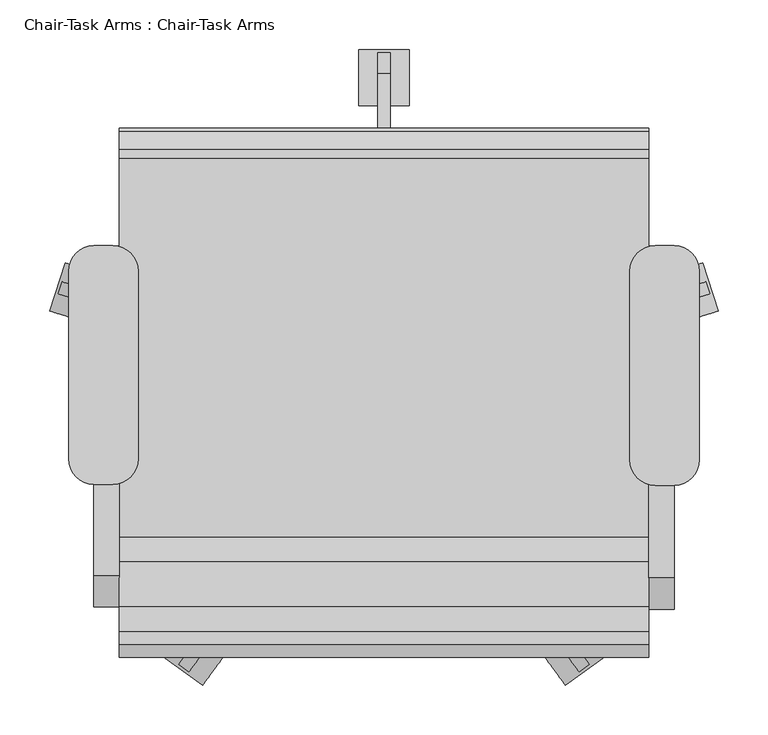
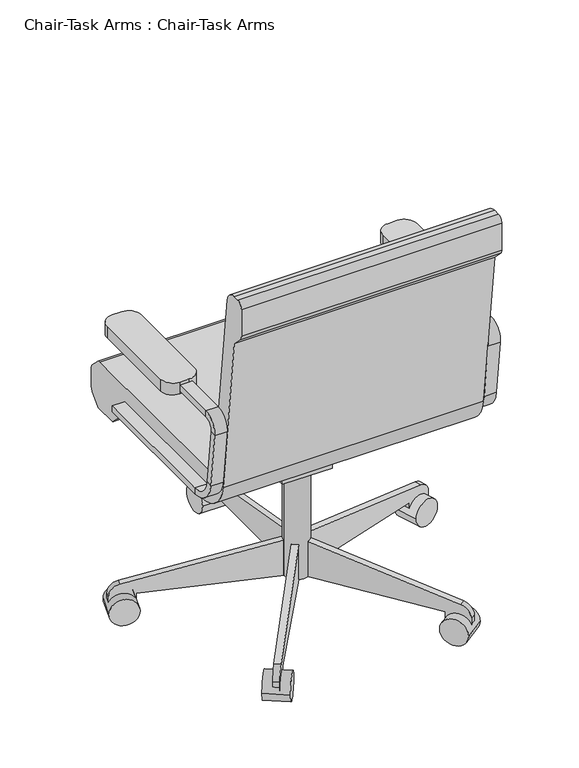
"""IFC4 building model written with IfcOpenShell, lengths in millimetres: furniture geometry, Chair-Task Arms : Chair-Task Arms."""

from ifc_helpers import new_model, si_unit, point, frame, frame_2d, origin, place, context, project, spatial, polyline, circle_curve, trimmed, segment, composite_curve, outline, extrude, source, transform, mapped, element, save
from ifc_brep_helpers import plane_surface, cylinder_surface, revolved_surface, advanced_brep


def chair_task_arms_chair_task_arms_fa5a08ef(model_context):
    return source(origin(), model_context, "Body", "SolidModel", [
        extrude(outline(composite_curve([segment(polyline([(433.0908197, -74.2028048), (414.0408197, -74.2028048)]), True, "CONTINUOUS"), segment(trimmed(circle_curve(frame_2d((414.0408197, -48.8028048)), 25.4), [point((414.0408197, -74.2028048))], [point((388.6408197, -48.8028048))], False, "CARTESIAN"), True, "CONTINUOUS"), segment(polyline([(388.6408197, -48.8028048), (388.6408197, 141.6319091)]), True, "CONTINUOUS"), segment(trimmed(circle_curve(frame_2d((414.0408197, 141.6319091)), 25.4), [point((388.6408197, 141.6319091))], [point((414.0408197, 167.0319091))], False, "CARTESIAN"), True, "CONTINUOUS"), segment(polyline([(414.0408197, 167.0319091), (433.0908197, 167.0319091)]), True, "CONTINUOUS"), segment(trimmed(circle_curve(frame_2d((433.0908197, 141.6319091)), 25.4), [point((433.0908197, 167.0319091))], [point((458.4908197, 141.6319091))], False, "CARTESIAN"), True, "CONTINUOUS"), segment(polyline([(458.4908197, 141.6319091), (458.4908197, -48.8028048)]), True, "CONTINUOUS"), segment(trimmed(circle_curve(frame_2d((433.0908197, -48.8028048)), 25.4), [point((458.4908197, -48.8028048))], [point((433.0908197, -74.2028048))], False, "CARTESIAN"), True, "CONTINUOUS")], self_intersect=False)), frame((0.0, 0.0, 596.9), z_axis=(0.0, 0.0, 1.0), x_axis=(1.0, 0.0, 0.0)), (0.0, 0.0, 1.0), 25.4),
        extrude(outline(composite_curve([segment(polyline([(-132.0591803, -73.1575984), (-151.1091803, -73.1575984)]), True, "CONTINUOUS"), segment(trimmed(circle_curve(frame_2d((-151.1091803, -47.7575984)), 25.4), [point((-151.1091803, -73.1575984))], [point((-176.5091803, -47.7575984))], False, "CARTESIAN"), True, "CONTINUOUS"), segment(polyline([(-176.5091803, -47.7575984), (-176.5091803, 141.6319091)]), True, "CONTINUOUS"), segment(trimmed(circle_curve(frame_2d((-151.1091803, 141.6319091)), 25.4), [point((-176.5091803, 141.6319091))], [point((-151.1091803, 167.0319091))], False, "CARTESIAN"), True, "CONTINUOUS"), segment(polyline([(-151.1091803, 167.0319091), (-132.0591803, 167.0319091)]), True, "CONTINUOUS"), segment(trimmed(circle_curve(frame_2d((-132.0591803, 141.6319091)), 25.4), [point((-132.0591803, 167.0319091))], [point((-106.6591803, 141.6319091))], False, "CARTESIAN"), True, "CONTINUOUS"), segment(polyline([(-106.6591803, 141.6319091), (-106.6591803, -47.7575984)]), True, "CONTINUOUS"), segment(trimmed(circle_curve(frame_2d((-132.0591803, -47.7575984)), 25.4), [point((-106.6591803, -47.7575984))], [point((-132.0591803, -73.1575984))], False, "CARTESIAN"), True, "CONTINUOUS")], self_intersect=False)), frame((0.0, 0.0, 596.9), z_axis=(0.0, 0.0, 1.0), x_axis=(1.0, 0.0, 0.0)), (0.0, 0.0, 1.0), 25.4),
        advanced_brep(
        [(-151.1091803, 167.0319091, 412.75), (-151.1091803, 167.0319091, 425.45), (-125.7091803, 167.0319091, 425.45), (-125.7091803, 167.0319091, 412.75), (-151.1091803, -126.2388651, 412.75), (-151.1091803, -126.2388651, 425.45), (-125.7091803, -126.2388651, 425.45), (-125.7091803, -126.2388651, 412.75), (-151.1091803, -170.3844094, 464.7064065), (-151.1091803, -182.9974221, 463.2225227), (-125.7091803, -170.3844094, 464.7064065), (-125.7091803, -182.9974221, 463.2225227), (-151.1091803, -196.7936301, 580.4902904), (-151.1091803, -184.1806174, 581.9741742), (-125.7091803, -184.1806174, 581.9741742), (-125.7091803, -196.7936301, 580.4902904), (-151.1091803, -165.2610984, 603.25), (-151.1091803, -165.2610984, 615.95), (-125.7091803, -165.2610984, 603.25), (-125.7091803, -165.2610984, 615.95), (-151.1091803, 18.9459016, 615.95), (-125.7091803, 18.9459016, 615.95), (-125.7091803, 18.9459016, 603.25), (-151.1091803, 18.9459016, 603.25)],
        [
            (0, 1),
            (1, 2),
            (2, 3),
            (3, 0),
            (0, 4),
            (4, 5),
            (5, 1),
            (5, 6),
            (6, 2),
            (6, 7),
            (7, 3),
            (7, 4),
            (8, 5, circle_curve(frame((-151.1091803, -126.2388651, 469.9), z_axis=(1.0, 0.0, 0.0), x_axis=(0.0, 0.0, -1.0)), 44.45)),
            (4, 9, circle_curve(frame((-151.1091803, -126.2388651, 469.9), z_axis=(-1.0, 0.0, 0.0), x_axis=(0.0, 0.0, -1.0)), 57.15)),
            (9, 8),
            (10, 6, circle_curve(frame((-125.7091803, -126.2388651, 469.9), z_axis=(1.0, 0.0, 0.0), x_axis=(0.0, 0.0, -1.0)), 44.45)),
            (8, 10),
            (11, 7, circle_curve(frame((-125.7091803, -126.2388651, 469.9), z_axis=(1.0, 0.0, 0.0), x_axis=(0.0, 0.0, -1.0)), 57.15)),
            (10, 11),
            (11, 9),
            (9, 12),
            (12, 13),
            (13, 8),
            (13, 14),
            (14, 10),
            (14, 15),
            (15, 11),
            (15, 12),
            (16, 13, circle_curve(frame((-151.1091803, -165.2610984, 584.2), z_axis=(1.0, 0.0, 0.0), x_axis=(0.0, -0.9931506043228768, -0.11684124756739202)), 19.05)),
            (12, 17, circle_curve(frame((-151.1091803, -165.2610984, 584.2), z_axis=(-1.0, 0.0, 0.0), x_axis=(0.0, -0.9931506043228768, -0.11684124756739202)), 31.75)),
            (17, 16),
            (18, 14, circle_curve(frame((-125.7091803, -165.2610984, 584.2), z_axis=(1.0, 0.0, 0.0), x_axis=(0.0, -0.9931506043228768, -0.11684124756739202)), 19.05)),
            (16, 18),
            (19, 15, circle_curve(frame((-125.7091803, -165.2610984, 584.2), z_axis=(1.0, 0.0, 0.0), x_axis=(0.0, -0.9931506043228768, -0.11684124756739202)), 31.75)),
            (18, 19),
            (19, 17),
            (20, 21),
            (21, 22),
            (22, 23),
            (23, 20),
            (17, 20),
            (23, 16),
            (22, 18),
            (21, 19),
        ],
        [
            plane_surface(frame((-152.608212, 167.0319091, 419.1), z_axis=(0.0, 1.0, 0.0), x_axis=(0.0, 0.0, -1.0))),
            plane_surface(frame((-151.1091803, 167.0319091, 412.75), z_axis=(-1.0, 0.0, 0.0), x_axis=(0.0, -1.0, 0.0))),
            plane_surface(frame((-151.1091803, 167.0319091, 425.45), z_axis=(0.0, 0.0, 1.0), x_axis=(0.0, -1.0, 0.0))),
            plane_surface(frame((-125.7091803, 167.0319091, 425.45), z_axis=(1.0, 0.0, 0.0), x_axis=(0.0, -1.0, 0.0))),
            plane_surface(frame((-125.7091803, 167.0319091, 412.75), z_axis=(0.0, 0.0, -1.0), x_axis=(0.0, -1.0, 0.0))),
            plane_surface(frame((-151.1091803, -126.2388651, 469.9), z_axis=(-1.0, 0.0, 0.0), x_axis=(0.0, 0.0, -1.0))),
            revolved_surface(polyline([(-151.1091803, -126.2388651, 425.45), (-125.7091803, -126.2388651, 425.45)]), (-138.4091803, -126.2388651, 469.9), (-1.0, 0.0, 0.0)),
            plane_surface(frame((-125.7091803, -126.2388651, 469.9), z_axis=(1.0, 0.0, 0.0), x_axis=(0.0, 0.0, -1.0))),
            cylinder_surface(frame((-138.4091803, -126.2388651, 469.9), z_axis=(-1.0, 0.0, 0.0), x_axis=(0.0, 0.0, -1.0)), 57.15),
            plane_surface(frame((-151.1091803, -182.9974221, 463.2225227), z_axis=(-1.0, 0.0, 0.0), x_axis=(0.0, -0.1168412475673856, 0.9931506043228776))),
            plane_surface(frame((-151.1091803, -170.3844094, 464.7064065), z_axis=(0.0, 0.9931506043228776, 0.1168412475673856), x_axis=(0.0, -0.1168412475673856, 0.9931506043228776))),
            plane_surface(frame((-125.7091803, -170.3844094, 464.7064065), z_axis=(1.0, 0.0, 0.0), x_axis=(0.0, -0.1168412475673856, 0.9931506043228776))),
            plane_surface(frame((-125.7091803, -182.9974221, 463.2225227), z_axis=(0.0, -0.9931506043228776, -0.1168412475673856), x_axis=(0.0, -0.1168412475673856, 0.9931506043228776))),
            plane_surface(frame((-151.1091803, -165.2610984, 584.2), z_axis=(-1.0, 0.0, 0.0), x_axis=(0.0, -0.9931506043228768, -0.11684124756739202))),
            revolved_surface(polyline([(-151.1091803, -184.1806174123508, 581.9741742338413), (-125.7091803, -184.1806174123508, 581.9741742338413)]), (-138.4091803, -165.2610984, 584.2), (-1.0, 0.0, 0.0)),
            plane_surface(frame((-125.7091803, -165.2610984, 584.2), z_axis=(1.0, 0.0, 0.0), x_axis=(0.0, -0.9931506043228768, -0.11684124756739202))),
            cylinder_surface(frame((-138.4091803, -165.2610984, 584.2), z_axis=(-1.0, 0.0, 0.0), x_axis=(0.0, -0.9931506043228768, -0.11684124756739202)), 31.75),
            plane_surface(frame((-152.608212, 18.9459016, 609.6), z_axis=(0.0, 1.0, 0.0), x_axis=(0.0, 0.0, 1.0))),
            plane_surface(frame((-151.1091803, -165.2610984, 615.95), z_axis=(-1.0, 0.0, 0.0), x_axis=(0.0, 1.0, 0.0))),
            plane_surface(frame((-151.1091803, -165.2610984, 603.25), z_axis=(0.0, 0.0, -1.0), x_axis=(0.0, 1.0, 0.0))),
            plane_surface(frame((-125.7091803, -165.2610984, 603.25), z_axis=(1.0, 0.0, 0.0), x_axis=(0.0, 1.0, 0.0))),
            plane_surface(frame((-125.7091803, -165.2610984, 615.95), z_axis=(0.0, 0.0, 1.0), x_axis=(0.0, 1.0, 0.0))),
        ],
        [
            (0, [[1, 2, 3, 4]]),
            (1, [[-1, 5, 6, 7]]),
            (2, [[-2, -7, 8, 9]]),
            (3, [[-3, -9, 10, 11]]),
            (4, [[-4, -11, 12, -5]]),
            (5, [[13, -6, 14, 15]]),
            (6, [[16, -8, -13, 17]]),
            (7, [[18, -10, -16, 19]]),
            (8, [[-14, -12, -18, 20]]),
            (9, [[-15, 21, 22, 23]]),
            (10, [[-17, -23, 24, 25]]),
            (11, [[-19, -25, 26, 27]]),
            (12, [[-20, -27, 28, -21]]),
            (13, [[29, -22, 30, 31]]),
            (14, [[32, -24, -29, 33]]),
            (15, [[34, -26, -32, 35]]),
            (16, [[-30, -28, -34, 36]]),
            (17, [[37, 38, 39, 40]]),
            (18, [[-31, 41, -40, 42]]),
            (19, [[-33, -42, -39, 43]]),
            (20, [[-35, -43, -38, 44]]),
            (21, [[-36, -44, -37, -41]]),
        ],
    ),
        advanced_brep(
        [(433.0908197, 167.0319091, 425.45), (433.0908197, 167.0319091, 412.75), (407.6908197, 167.0319091, 412.75), (407.6908197, 167.0319091, 425.45), (433.0908197, -128.329278, 425.45), (433.0908197, -128.329278, 412.75), (407.6908197, -128.329278, 412.75), (407.6908197, -128.329278, 425.45), (433.0908197, -185.0878351, 463.2225227), (433.0908197, -172.4748224, 464.7064065), (407.6908197, -185.0878351, 463.2225227), (407.6908197, -172.4748224, 464.7064065), (433.0908197, -186.2710303, 581.9741742), (433.0908197, -198.884043, 580.4902904), (407.6908197, -198.884043, 580.4902904), (407.6908197, -186.2710303, 581.9741742), (433.0908197, -167.3515113, 615.95), (433.0908197, -167.3515113, 603.25), (407.6908197, -167.3515113, 615.95), (407.6908197, -167.3515113, 603.25), (433.0908197, 18.9459016, 603.25), (407.6908197, 18.9459016, 603.25), (407.6908197, 18.9459016, 615.95), (433.0908197, 18.9459016, 615.95)],
        [
            (0, 1),
            (1, 2),
            (2, 3),
            (3, 0),
            (0, 4),
            (4, 5),
            (5, 1),
            (5, 6),
            (6, 2),
            (6, 7),
            (7, 3),
            (7, 4),
            (8, 5, circle_curve(frame((433.0908197, -128.329278, 469.9), z_axis=(1.0, 0.0, 0.0), x_axis=(0.0, 0.0, -1.0)), 57.15)),
            (4, 9, circle_curve(frame((433.0908197, -128.329278, 469.9), z_axis=(-1.0, 0.0, 0.0), x_axis=(0.0, 0.0, -1.0)), 44.45)),
            (9, 8),
            (10, 6, circle_curve(frame((407.6908197, -128.329278, 469.9), z_axis=(1.0, 0.0, 0.0), x_axis=(0.0, 0.0, -1.0)), 57.15)),
            (8, 10),
            (11, 7, circle_curve(frame((407.6908197, -128.329278, 469.9), z_axis=(1.0, 0.0, 0.0), x_axis=(0.0, 0.0, -1.0)), 44.45)),
            (10, 11),
            (11, 9),
            (9, 12),
            (12, 13),
            (13, 8),
            (13, 14),
            (14, 10),
            (14, 15),
            (15, 11),
            (15, 12),
            (16, 13, circle_curve(frame((433.0908197, -167.3515113, 584.2), z_axis=(1.0, 0.0, 0.0), x_axis=(0.0, -0.9931506043228767, -0.1168412475673929)), 31.75)),
            (12, 17, circle_curve(frame((433.0908197, -167.3515113, 584.2), z_axis=(-1.0, 0.0, 0.0), x_axis=(0.0, -0.9931506043228767, -0.1168412475673929)), 19.05)),
            (17, 16),
            (18, 14, circle_curve(frame((407.6908197, -167.3515113, 584.2), z_axis=(1.0, 0.0, 0.0), x_axis=(0.0, -0.9931506043228767, -0.1168412475673929)), 31.75)),
            (16, 18),
            (19, 15, circle_curve(frame((407.6908197, -167.3515113, 584.2), z_axis=(1.0, 0.0, 0.0), x_axis=(0.0, -0.9931506043228767, -0.1168412475673929)), 19.05)),
            (18, 19),
            (19, 17),
            (20, 21),
            (21, 22),
            (22, 23),
            (23, 20),
            (17, 20),
            (23, 16),
            (22, 18),
            (21, 19),
        ],
        [
            plane_surface(frame((406.191788, 167.0319091, 419.1), z_axis=(0.0, 1.0, 0.0), x_axis=(0.0, 0.0, -1.0))),
            plane_surface(frame((433.0908197, 167.0319091, 425.45), z_axis=(1.0, 0.0, 0.0), x_axis=(0.0, -1.0, 0.0))),
            plane_surface(frame((433.0908197, 167.0319091, 412.75), z_axis=(0.0, 0.0, -1.0), x_axis=(0.0, -1.0, 0.0))),
            plane_surface(frame((407.6908197, 167.0319091, 412.75), z_axis=(-1.0, 0.0, 0.0), x_axis=(0.0, -1.0, 0.0))),
            plane_surface(frame((407.6908197, 167.0319091, 425.45), z_axis=(0.0, 0.0, 1.0), x_axis=(0.0, -1.0, 0.0))),
            plane_surface(frame((433.0908197, -128.329278, 469.9), z_axis=(1.0, 0.0, 0.0), x_axis=(0.0, 0.0, -1.0))),
            cylinder_surface(frame((420.3908197, -128.329278, 469.9), z_axis=(-1.0, 0.0, 0.0), x_axis=(0.0, 0.0, -1.0)), 57.15),
            plane_surface(frame((407.6908197, -128.329278, 469.9), z_axis=(-1.0, 0.0, 0.0), x_axis=(0.0, 0.0, -1.0))),
            revolved_surface(polyline([(407.6908197, -128.329278, 425.45), (433.0908197, -128.329278, 425.45)]), (420.3908197, -128.329278, 469.9), (-1.0, 0.0, 0.0)),
            plane_surface(frame((433.0908197, -172.4748224, 464.7064065), z_axis=(1.0, 0.0, 0.0), x_axis=(0.0, -0.11684124756738626, 0.9931506043228775))),
            plane_surface(frame((433.0908197, -185.0878351, 463.2225227), z_axis=(0.0, -0.9931506043228775, -0.11684124756738655), x_axis=(0.0, -0.11684124756738655, 0.9931506043228775))),
            plane_surface(frame((407.6908197, -185.0878351, 463.2225227), z_axis=(-1.0, 0.0, 0.0), x_axis=(0.0, -0.11684124756738626, 0.9931506043228775))),
            plane_surface(frame((407.6908197, -172.4748224, 464.7064065), z_axis=(0.0, 0.9931506043228775, 0.11684124756738626), x_axis=(0.0, -0.11684124756738626, 0.9931506043228775))),
            plane_surface(frame((433.0908197, -167.3515113, 584.2), z_axis=(1.0, 0.0, 0.0), x_axis=(0.0, -0.9931506043228767, -0.1168412475673929))),
            cylinder_surface(frame((420.3908197, -167.3515113, 584.2), z_axis=(-1.0, 0.0, 0.0), x_axis=(0.0, -0.9931506043228767, -0.1168412475673929)), 31.75),
            plane_surface(frame((407.6908197, -167.3515113, 584.2), z_axis=(-1.0, 0.0, 0.0), x_axis=(0.0, -0.9931506043228767, -0.1168412475673929))),
            revolved_surface(polyline([(407.6908197, -186.2710303123508, 581.9741742338412), (433.0908197, -186.2710303123508, 581.9741742338412)]), (420.3908197, -167.3515113, 584.2), (-1.0, 0.0, 0.0)),
            plane_surface(frame((406.191788, 18.9459016, 609.6), z_axis=(0.0, 1.0, 0.0), x_axis=(0.0, 0.0, 1.0))),
            plane_surface(frame((433.0908197, -167.3515113, 603.25), z_axis=(1.0, 0.0, 0.0), x_axis=(0.0, 1.0, 0.0))),
            plane_surface(frame((433.0908197, -167.3515113, 615.95), z_axis=(0.0, 0.0, 1.0), x_axis=(0.0, 1.0, 0.0))),
            plane_surface(frame((407.6908197, -167.3515113, 615.95), z_axis=(-1.0, 0.0, 0.0), x_axis=(0.0, 1.0, 0.0))),
            plane_surface(frame((407.6908197, -167.3515113, 603.25), z_axis=(0.0, 0.0, -1.0), x_axis=(0.0, 1.0, 0.0))),
        ],
        [
            (0, [[1, 2, 3, 4]]),
            (1, [[-1, 5, 6, 7]]),
            (2, [[-2, -7, 8, 9]]),
            (3, [[-3, -9, 10, 11]]),
            (4, [[-4, -11, 12, -5]]),
            (5, [[13, -6, 14, 15]]),
            (6, [[16, -8, -13, 17]]),
            (7, [[18, -10, -16, 19]]),
            (8, [[-14, -12, -18, 20]]),
            (9, [[-15, 21, 22, 23]]),
            (10, [[-17, -23, 24, 25]]),
            (11, [[-19, -25, 26, 27]]),
            (12, [[-20, -27, 28, -21]]),
            (13, [[29, -22, 30, 31]]),
            (14, [[32, -24, -29, 33]]),
            (15, [[34, -26, -32, 35]]),
            (16, [[-30, -28, -34, 36]]),
            (17, [[37, 38, 39, 40]]),
            (18, [[-31, 41, -40, 42]]),
            (19, [[-33, -42, -39, 43]]),
            (20, [[-35, -43, -38, 44]]),
            (21, [[-36, -44, -37, -41]]),
        ],
    ),
        extrude(outline(composite_curve([segment(trimmed(circle_curve(frame_2d((140.9908197, 18.9459016)), 25.4), [point((115.5908197, 18.9459016))], [point((166.3908197, 18.9459016))], False, "CARTESIAN"), True, "CONTINUOUS"), segment(trimmed(circle_curve(frame_2d((140.9908197, 18.9459016)), 25.4), [point((166.3908197, 18.9459016))], [point((115.5908197, 18.9459016))], False, "CARTESIAN"), True, "CONTINUOUS")], self_intersect=False)), frame((0.0, 0.0, 53.5835944), z_axis=(0.0, 0.0, 1.0), x_axis=(1.0, 0.0, 0.0)), (0.0, 0.0, 1.0), 330.5914056),
        extrude(outline(composite_curve([segment(trimmed(circle_curve(frame_2d((0.0, -28.2002727)), 28.2002727), [point((0.0, -56.4005455))], [point((0.0, 0.0))], False, "CARTESIAN"), True, "CONTINUOUS"), segment(trimmed(circle_curve(frame_2d((0.0, -28.2002727)), 28.2002727), [point((0.0, 0.0))], [point((0.0, -56.4005455))], False, "CARTESIAN"), True, "CONTINUOUS")], self_intersect=False)), frame((477.6203484, 101.6163254, 28.1835944), z_axis=(-0.3090169943749423, 0.9510565162951553, 0.0), x_axis=(0.0, 0.0, 1.0)), (0.0, 0.0, 1.0), 50.8),
        extrude(outline(composite_curve([segment(polyline([(-25.4, 0.0), (0.0, 0.0), (0.0, -50.8), (-24.303053, -50.8)]), True, "CONTINUOUS"), segment(trimmed(circle_curve(frame_2d((-24.303053, -25.4)), 25.4), [point((-24.303053, -50.8))], [point((-49.3171699, -29.8106637))], False, "CARTESIAN"), True, "CONTINUOUS"), segment(polyline([(-49.3171699, -29.8106637), (-101.6, 266.7), (-101.6, 292.1), (-25.4, 292.1), (-25.4, 0.0)]), True, "CONTINUOUS")], self_intersect=False)), frame((420.756686, 103.1705568, 28.1835944), z_axis=(-0.3090169943749423, 0.9510565162951553, 0.0), x_axis=(0.0, 0.0, -1.0)), (0.0, 0.0, 1.0), 12.7),
        extrude(outline(composite_curve([segment(trimmed(circle_curve(frame_2d((0.0, -28.2002727)), 28.2002727), [point((0.0, -56.4005455))], [point((0.0, 0.0))], False, "CARTESIAN"), True, "CONTINUOUS"), segment(trimmed(circle_curve(frame_2d((0.0, -28.2002727)), 28.2002727), [point((0.0, 0.0))], [point((0.0, -56.4005455))], False, "CARTESIAN"), True, "CONTINUOUS")], self_intersect=False)), frame((323.63931, -275.6612394, 28.1835944), z_axis=(0.8090169943749499, 0.5877852522924699, 0.0), x_axis=(0.0, 0.0, 1.0)), (0.0, 0.0, 1.0), 50.8),
        extrude(outline(composite_curve([segment(polyline([(-25.4, 0.0), (0.0, 0.0), (0.0, -50.8), (-24.303053, -50.8)]), True, "CONTINUOUS"), segment(trimmed(circle_curve(frame_2d((-24.303053, -25.3999999)), 25.4), [point((-24.303053, -50.8))], [point((-49.3171699, -29.8106636))], False, "CARTESIAN"), True, "CONTINUOUS"), segment(polyline([(-49.3171699, -29.8106636), (-101.6, 266.7), (-101.6, 292.1), (-25.4, 292.1), (-25.4, 0.0)]), True, "CONTINUOUS")], self_intersect=False)), frame((307.545634, -221.1003988, 28.1835944), z_axis=(0.8090169943749499, 0.5877852522924699, 0.0), x_axis=(0.0, 0.0, -1.0)), (0.0, 0.0, 1.0), 12.7),
        extrude(outline(composite_curve([segment(trimmed(circle_curve(frame_2d((0.0, -28.2002727)), 28.2002727), [point((0.0, -56.4005455))], [point((0.0, 0.0))], False, "CARTESIAN"), True, "CONTINUOUS"), segment(trimmed(circle_curve(frame_2d((0.0, -28.2002727)), 28.2002727), [point((0.0, 0.0))], [point((0.0, -56.4005455))], False, "CARTESIAN"), True, "CONTINUOUS")], self_intersect=False)), frame((-41.6576707, -275.6612394, 28.1835944), z_axis=(-0.8090169943749458, 0.5877852522924754, 0.0), x_axis=(0.0, 0.0, -1.0)), (0.0, 0.0, 1.0), 50.8),
        extrude(outline(composite_curve([segment(polyline([(25.4, 0.0), (25.4, 292.1), (101.6, 292.1), (101.6, 266.7), (49.3171699, -29.8106637)]), True, "CONTINUOUS"), segment(trimmed(circle_curve(frame_2d((24.303053, -25.3999999)), 25.4), [point((49.3171699, -29.8106637))], [point((24.303053, -50.8))], False, "CARTESIAN"), True, "CONTINUOUS"), segment(polyline([(24.303053, -50.8), (0.0, -50.8), (0.0, 0.0), (25.4, 0.0)]), True, "CONTINUOUS")], self_intersect=False)), frame((-25.5639946, -221.1003988, 28.1835944), z_axis=(-0.8090169943749459, 0.5877852522924754, 0.0), x_axis=(0.0, 0.0, 1.0)), (0.0, 0.0, 1.0), 12.7),
        extrude(outline(composite_curve([segment(trimmed(circle_curve(frame_2d((0.0, -28.2002727)), 28.2002727), [point((0.0, -56.4005454))], [point((0.0, 0.0))], False, "CARTESIAN"), True, "CONTINUOUS"), segment(trimmed(circle_curve(frame_2d((0.0, -28.2002727)), 28.2002727), [point((0.0, 0.0))], [point((0.0, -56.4005454))], False, "CARTESIAN"), True, "CONTINUOUS")], self_intersect=False)), frame((-195.638709, 101.6163254, 28.1835944), z_axis=(0.3090169943749487, 0.9510565162951532, 0.0), x_axis=(0.0, 0.0, -1.0)), (0.0, 0.0, 1.0), 50.8),
        extrude(outline(composite_curve([segment(polyline([(25.4, 0.0), (25.4, 292.1000001), (101.6, 292.1000001), (101.6, 266.7), (49.3171699, -29.8106636)]), True, "CONTINUOUS"), segment(trimmed(circle_curve(frame_2d((24.303053, -25.4)), 25.4), [point((49.3171699, -29.8106636))], [point((24.303053, -50.8))], False, "CARTESIAN"), True, "CONTINUOUS"), segment(polyline([(24.303053, -50.8), (0.0, -50.8), (0.0, 0.0), (25.4, 0.0)]), True, "CONTINUOUS")], self_intersect=False)), frame((-138.7750467, 103.1705568, 28.1835944), z_axis=(0.3090169943749487, 0.9510565162951532, 0.0), x_axis=(0.0, 0.0, 1.0)), (0.0, 0.0, 1.0), 12.7),
        extrude(outline(composite_curve([segment(trimmed(circle_curve(frame_2d((336.4459016, 28.1835944)), 28.2002727), [point((308.2456289, 28.1835944))], [point((364.6461744, 28.1835944))], False, "CARTESIAN"), True, "CONTINUOUS"), segment(trimmed(circle_curve(frame_2d((336.4459016, 28.1835944)), 28.2002727), [point((364.6461744, 28.1835944))], [point((308.2456289, 28.1835944))], False, "CARTESIAN"), True, "CONTINUOUS")], self_intersect=False)), frame((115.5908197, 0.0, 0.0), z_axis=(1.0, 0.0, 0.0), x_axis=(0.0, 1.0, 0.0)), (0.0, 0.0, 1.0), 50.8),
        extrude(outline(composite_curve([segment(polyline([(311.0459016, 53.5835944), (18.9459016, 53.5835944), (18.9459016, 129.7835944), (44.3459016, 129.7835944), (340.8565654, 77.5007643)]), True, "CONTINUOUS"), segment(trimmed(circle_curve(frame_2d((336.4459016, 52.4866474)), 25.4), [point((340.8565654, 77.5007643))], [point((361.8459016, 52.4866474))], False, "CARTESIAN"), True, "CONTINUOUS"), segment(polyline([(361.8459016, 52.4866474), (361.8459016, 28.1835944), (311.0459016, 28.1835944), (311.0459016, 53.5835944)]), True, "CONTINUOUS")], self_intersect=False)), frame((134.6408197, 0.0, 0.0), z_axis=(1.0, 0.0, 0.0), x_axis=(0.0, 1.0, 0.0)), (0.0, 0.0, 1.0), 12.7),
        extrude(outline(polyline([(69.7459016, 383.7835944), (69.7459016, 371.0835944), (18.9459016, 283.0954134), (-19.1540984, 283.0954134), (-19.1540984, 383.7835944), (69.7459016, 383.7835944)])), frame((90.1908197, 0.0, 0.0), z_axis=(1.0, 0.0, 0.0), x_axis=(0.0, 1.0, 0.0)), (0.0, 0.0, 1.0), 101.6),
        extrude(outline(composite_curve([segment(polyline([(-126.2050455, 457.2), (255.0102301, 457.2)]), True, "CONTINUOUS"), segment(trimmed(circle_curve(frame_2d((255.0102301, 444.5)), 12.7), [point((255.0102301, 457.2))], [point((263.9604301, 453.510212))], False, "CARTESIAN"), True, "CONTINUOUS"), segment(polyline([(263.9604301, 453.510212), (281.8961016, 435.6939999)]), True, "CONTINUOUS"), segment(trimmed(circle_curve(frame_2d((272.9459016, 426.6837879)), 12.7), [point((281.8961016, 435.6939999))], [point((285.6459016, 426.6837879))], False, "CARTESIAN"), True, "CONTINUOUS"), segment(polyline([(285.6459016, 426.6837879), (285.6459016, 391.6405184)]), True, "CONTINUOUS"), segment(trimmed(circle_curve(frame_2d((260.2459016, 391.6405184)), 25.4), [point((285.6459016, 391.6405184))], [point((278.2663256, 373.7401184))], False, "CARTESIAN"), True, "CONTINUOUS"), segment(polyline([(278.2663256, 373.7401184), (260.2470284, 355.6), (209.4470284, 355.6), (181.0744602, 383.7835944), (-107.1089978, 383.7835944)]), True, "CONTINUOUS"), segment(trimmed(circle_curve(frame_2d((-107.1089978, 459.9835944)), 76.2), [point((-107.1089978, 383.7835944))], [point((-182.7870738, 451.0802913))], False, "CARTESIAN"), True, "CONTINUOUS"), segment(polyline([(-182.7870738, 451.0802913), (-222.3540984, 787.4), (-244.0343545, 809.0802561)]), True, "CONTINUOUS"), segment(trimmed(circle_curve(frame_2d((-235.0540984, 818.0605122)), 12.7), [point((-244.0343545, 809.0802561))], [point((-247.7540984, 818.0605122))], False, "CARTESIAN"), True, "CONTINUOUS"), segment(polyline([(-247.7540984, 818.0605122), (-247.7540984, 876.3)]), True, "CONTINUOUS"), segment(trimmed(circle_curve(frame_2d((-235.0540984, 876.3)), 12.7), [point((-247.7540984, 876.3))], [point((-235.0540984, 889.0))], False, "CARTESIAN"), True, "CONTINUOUS"), segment(polyline([(-235.0540984, 889.0), (-222.1789239, 889.0)]), True, "CONTINUOUS"), segment(trimmed(circle_curve(frame_2d((-222.1789239, 863.6)), 25.4), [point((-222.1789239, 889.0))], [point((-196.9528985, 866.5677677))], False, "CARTESIAN"), True, "CONTINUOUS"), segment(polyline([(-196.9528985, 866.5677677), (-151.4310708, 479.6322323)]), True, "CONTINUOUS"), segment(trimmed(circle_curve(frame_2d((-126.2050455, 482.6)), 25.4), [point((-151.4310708, 479.6322323))], [point((-126.2050455, 457.2))], True, "CARTESIAN"), True, "CONTINUOUS")], self_intersect=False)), frame((-125.7091803, 0.0, 0.0), z_axis=(1.0, 0.0, 0.0), x_axis=(0.0, 1.0, 0.0)), (0.0, 0.0, 1.0), 533.4),
    ])


if __name__ == "__main__":
    model = new_model("IFC4")
    model_context = context("Model", 3, world=origin())
    ifc_project = project(units=[si_unit("LENGTHUNIT", "METRE", prefix="MILLI")], contexts=[model_context])
    site = spatial("IfcSite", under=ifc_project)
    building = spatial("IfcBuilding", under=site)
    placement = place(None, origin())
    chair_task_arms_chair_task_arms_shape = chair_task_arms_chair_task_arms_fa5a08ef(model_context)
    element("IfcFurniture", 1, ObjectType="Chair-Task Arms : Chair-Task Arms", at=placement, inside=building, context=model_context, shape_type="MappedRepresentation", body=[
        mapped(chair_task_arms_chair_task_arms_shape, transform((0.0, 0.0, 0.0), x_axis=(1.0, 0.0, 0.0), y_axis=(0.0, 1.0, 0.0), z_axis=(0.0, 0.0, 1.0))),
    ])
    save(model, "model.ifc")

# Revit data of these elements
# Type "Chair-Task Arms : Chair-Task Arms"
#   Assembly Code = "E2020200"
#   Base Material = Plastic - Black
#   Caster Material = Plastic - Black
#   Seat/Back Material = Textile - Slate Blue
#   Default Elevation = 0
# Element 1 (IfcFurniture, "Chair-Task Arms : Chair-Task Arms")
#   Materials on its faces: "Plastic - Black", "Textile - Slate Blue"
# Materials
#   "Plastic - Black": colour RGB 0 0 0, transparency 0
#   "Textile - Slate Blue": colour RGB 98 102 118, transparency 0
